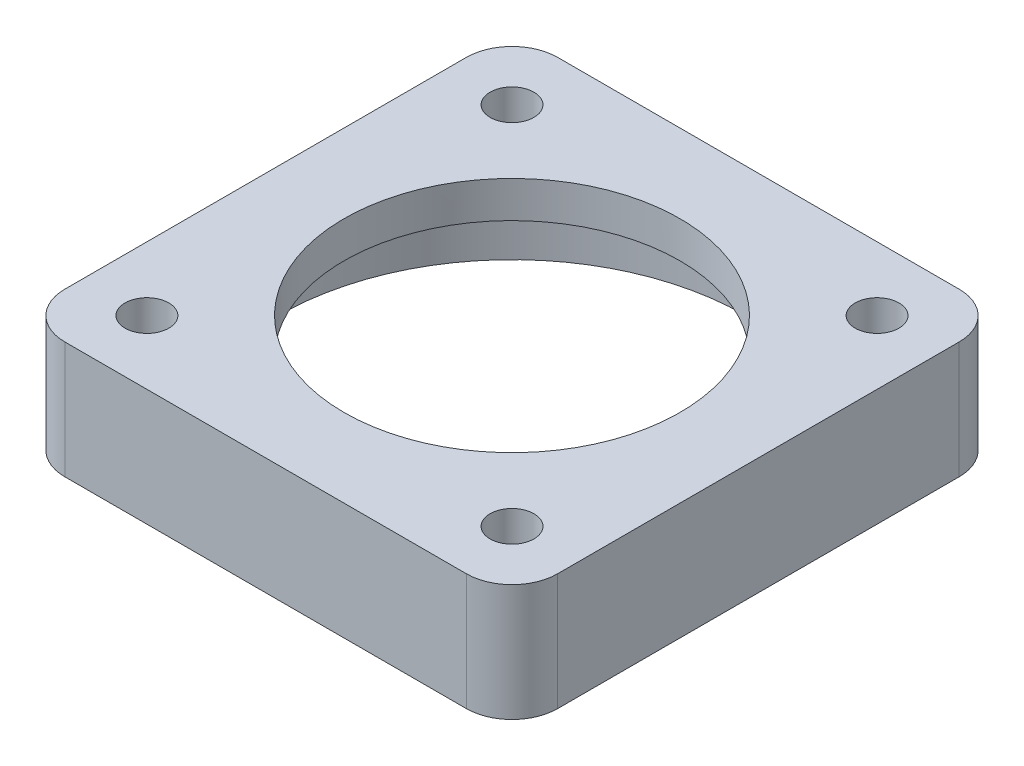
SolidWorks part; units mm, degrees
material "Plain Carbon Steel"
ref_plane "Front Plane" through (0, 0, 0) normal (0, 0, 1) x (1, 0, 0)
ref_plane "Top Plane" through (0, 0, 0) normal (0, 1, 0) x (1, 0, 0)
ref_plane "Right Plane" through (0, 0, 0) normal (1, 0, 0) x (0, 0, -1)
sketch "Base Plate Profile" plane through (0, 0, 0) normal (0, 1, 0) x (1, 0, 0)
  line L0 (0, 111.2234) -> (0, -96.5426) construction
  line L1 (218.617, 0) -> (-202.0213, 0) construction
  line L3 (-55, 67.5) -> (55, 67.5)
  line L4 (-67.5, 55) -> (-67.5, -55)
  line L5 (-55, -67.5) -> (55, -67.5)
  line L6 (67.5, 55) -> (67.5, -55)
  line L7 (-67.5, 67.5) -> (67.5, -67.5) construction
  line L8 (-67.5, -67.5) -> (67.5, 67.5) construction
  arc A0 (-67.5, -55) -> (-55, -67.5) centre (-55, -55) ccw
  arc A1 (55, -67.5) -> (67.5, -55) centre (55, -55) ccw
  arc A2 (67.5, 55) -> (55, 67.5) centre (55, 55) ccw
  arc A3 (-67.5, 55) -> (-55, 67.5) centre (-55, 55) cw
  circle A4 centre (-50, 50) radius 6
  circle A5 centre (50, 50) radius 6
  circle A6 centre (50, -50) radius 6
  circle A7 centre (-50, -50) radius 6
  point P5 (0, 0)
  dimension "D3" = 12.5
  dimension "D6" = 12
  dimension "D1" = 135
  dimension "D2" = 135
  dimension "D4" = 50
  dimension "D5" = 50
extrude "Base Plate 135x135x32" add sketch "Base Plate Profile" along normal blind 32
sketch "Through Bore Profile" plane through (0, 32, 0) normal (0, 1, 0) x (1, 0, 0)
  circle A0 centre (0, 0) radius 46
  dimension "D1" = 92
extrude "Through Bore Ø92" cut sketch "Through Bore Profile" against normal up to next contours A0
sketch "Counterbore Profile" plane through (0, 0, 0) normal (0, -1, 0) x (-1, 0, 0)
  circle A0 centre (0, 0) radius 64
  dimension "D1" = 128
extrude "Counterbore Ø128x22" cut sketch "Counterbore Profile" against normal blind 22
